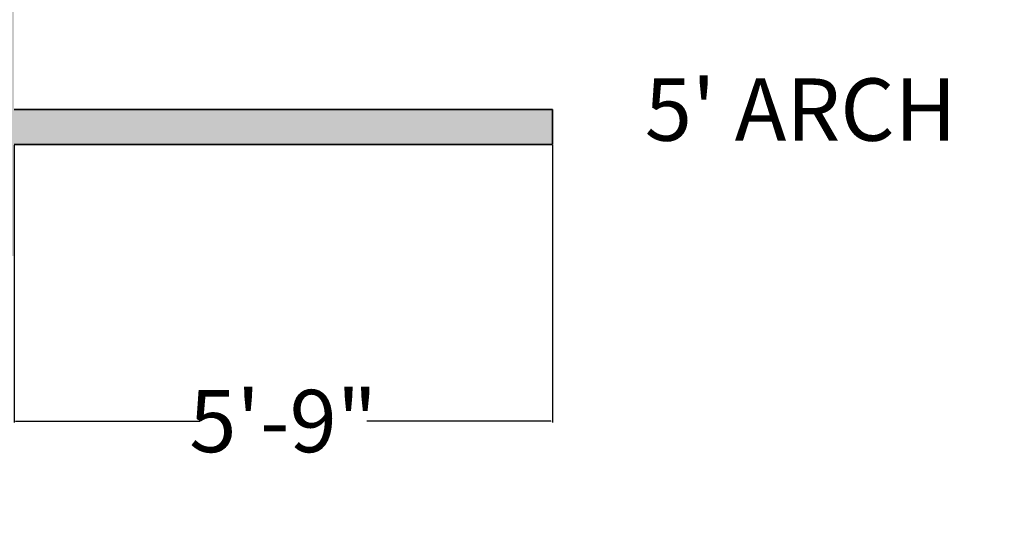
# Model space of a CAD drawing. Units: inches. Extents: x 638 to 1303, y 1 to 699.
# Tile 6 of 21: x 855 to 982, y 156 to 223. Entities that reach past the tile are written whole.
import ezdxf

# ---------------------------------------------------------------- set-up
doc = ezdxf.new("R2010")
doc.units = ezdxf.units.IN
doc.header["$MEASUREMENT"] = 0
for name, color, linetype, lineweight in [('A-ANNO-DIMS', 2, 'Continuous', 18), ('A-ANNO-TEXT', 7, 'Continuous', 18), ('A-WALL', 7, 'Continuous', 35)]:
    doc.layers.add(name, color=color, linetype=linetype, lineweight=lineweight)
doc.layers.add('A-WALL-PATT', color=143, linetype='Continuous', lineweight=13, true_color=0x7aafdf)
doc.styles.get("Standard").update_dxf_attribs({"font": 'arial.ttf'})
doc.dimstyles.get("Standard").update_dxf_attribs({"dimtxt": 8, "dimasz": 0.18, "dimexe": 0.18, "dimexo": 0.0625, "dimgap": 0.09, "dimtad": 0, "dimtih": 1, "dimtoh": 1, "dimdec": 4, "dimzin": 0, "dimdsep": 46, "dimlunit": 3, "dimtxsty": 'Standard', "dimcen": 0.09, "dimadec": 0, "dimazin": 0, "dimtfac": 1, "dimtdec": 4, "dimtofl": 0, "dimtmove": 0, "dimatfit": 3, "dimfxl": 1, "dimtolj": 1, "dimtzin": 0, "dimarcsym": 0})

# ---------------------------------------------------------------- blocks, each defined once
blk = doc.blocks.new('*D61')
at = {"layer": 'A-ANNO-DIMS', "color": 0, "lineweight": -2, "transparency": 16777216}
for p, q in [((854.74, 206.76), (854.74, 171.14)), ((923.85, 206.76), (923.85, 171.14)), ((854.92, 171.32), (878.57, 171.32)), ((923.67, 171.32), (900.02, 171.32))]:
    blk.add_line(p, q, dxfattribs=at)
at = {"layer": 'A-ANNO-DIMS', "color": 0, "transparency": 16777216}
for points in [[(854.92, 171.35), (854.92, 171.29), (854.74, 171.32)], [(923.67, 171.35), (923.67, 171.29), (923.85, 171.32)]]:
    blk.add_solid(points, dxfattribs=at)
at = {"layer": 'Defpoints', "color": 0, "transparency": 16777216}
for p in [(854.74, 206.82), (923.85, 206.82), (854.74, 171.32)]:
    blk.add_point(p, dxfattribs=at)
at = {"layer": 'A-ANNO-DIMS', "color": 0, "transparency": 16777216, "insert": (889.29, 171.32), "char_height": 8, "attachment_point": 5}
blk.add_mtext('\\A1;5\'-9"', dxfattribs=at)

msp = doc.modelspace()

# ---------------------------------------------------------------- hatches: boundary and pattern name
at = {"layer": 'A-WALL-PATT'}
h = msp.add_hatch(color=256, dxfattribs=at)
h.dxf.hatch_style = 1
h.paths.add_polyline_path([(973.34524, 629.81895), (793.35541, 629.81895), (793.35541, 620.81895), (850.23798, 620.81895), (922.23798, 620.81895), (922.23798, 524.81895), (908.94335, 524.81895), (908.94335, 520.31895), (926.73798, 520.31895), (926.73798, 544.31895), (979.3571, 544.31895), (979.3571, 548.81895), (926.73798, 548.81895), (926.73798, 620.81895), (973.34524, 620.81895)])
h.paths.add_polyline_path([(758.35541, 629.81895), (697.23798, 629.81895), (697.23798, 586.77451), (706.23798, 586.77451), (706.23798, 620.81895), (758.35541, 620.81895)])
h.paths.add_polyline_path([(1075.85281, 629.81895), (1003.34524, 629.81895), (1003.34524, 620.81895), (1046.73798, 620.81895), (1046.73798, 560.81895), (1046.73798, 548.81895), (1026.3571, 548.81895), (1026.3571, 544.31895), (1046.73798, 544.31895), (1046.73798, 486.87457), (1051.23798, 486.87457), (1051.23798, 556.31895), (1162.89753, 556.31895), (1162.89753, 560.81895), (1051.23798, 560.81895), (1051.23798, 620.81895), (1075.85281, 620.81895)])
h.paths.add_polyline_path([(1228.23798, 629.81895), (1105.85281, 629.81895), (1105.85281, 620.81895), (1219.23798, 620.81895), (1219.23798, 560.81895), (1197.89753, 560.81895), (1197.89753, 556.31895), (1219.23798, 556.31895), (1219.23798, 498.80084), (1228.23798, 498.80084)])
h.paths.add_polyline_path([(1051.23798, 439.87457), (1046.73798, 439.87457), (1046.73798, 407.81895), (1219.23798, 407.81895), (1219.23798, 381.66175), (1228.23798, 381.66175), (1228.23798, 451.80084), (1219.23798, 451.80084), (1219.23798, 412.31895), (1051.23798, 412.31895)])
h.paths.add_polyline_path([(1228.23798, 346.66175), (1219.23798, 346.66175), (1219.23798, 335.81895), (1046.73798, 335.81895), (1046.73798, 273.56895), (1051.23798, 273.56895), (1051.23798, 331.31895), (1219.23798, 331.31895), (1219.23798, 308.99654), (1228.23798, 308.99654)])
h.paths.add_polyline_path([(1228.23798, 261.99654), (1219.23798, 261.99654), (1219.23798, 211.31895), (1051.23798, 211.31895), (1051.23798, 226.56895), (1046.73798, 226.56895), (1046.73798, 211.31895), (983.84714, 211.31895), (983.84714, 206.81895), (1219.23798, 206.81895), (1219.23798, 166.83987), (1228.23798, 166.83987)])
h.paths.add_polyline_path([(1228.23798, 119.83987), (1219.23798, 119.83987), (1219.23798, 50.81895), (1197.89277, 50.81895), (1197.89277, 41.81895), (1228.23798, 41.81895)])
h.paths.add_polyline_path([(1162.89277, 50.81895), (1069.02949, 50.81895), (1069.02949, 41.81895), (1162.89277, 41.81895)])
h.paths.add_polyline_path([(1010.02949, 50.81895), (941.89631, 50.81895), (917.77455, 50.81895), (917.77455, 41.81895), (941.89631, 41.81895), (1010.02949, 41.81895)])
h.paths.add_polyline_path([(882.77455, 50.81895), (854.73798, 50.81895), (854.73798, 145.50379), (850.23798, 145.50379), (850.23798, 50.81895), (793.49755, 50.81895), (793.49755, 41.81895), (882.77455, 41.81895)])
h.paths.add_polyline_path([(746.49755, 50.81895), (706.23798, 50.81895), (706.23798, 96.57416), (697.23798, 96.57416), (697.23798, 41.81895), (746.49755, 41.81895)])
h.paths.add_polyline_path([(706.23798, 206.81895), (714.01165, 206.81895), (714.01165, 211.31895), (706.23798, 211.31895), (706.23798, 251.21966), (697.23798, 251.21966), (697.23798, 143.57416), (706.23798, 143.57416)])
h.paths.add_polyline_path([(923.84714, 211.31895), (854.73798, 211.31895), (854.73798, 397.8313), (850.23798, 397.8313), (850.23798, 388.31895), (747.9539, 388.31895), (747.9539, 383.81895), (850.23798, 383.81895), (850.23798, 311.81895), (706.23798, 311.81895), (706.23798, 342.78787), (697.23798, 342.78787), (697.23798, 281.21966), (706.23798, 281.21966), (706.23798, 307.31895), (850.23798, 307.31895), (850.23798, 211.31895), (749.01165, 211.31895), (749.01165, 206.81895), (850.23798, 206.81895), (850.23798, 192.50379), (854.73798, 192.50379), (854.73798, 206.81895), (923.84714, 206.81895)])
h.paths.add_polyline_path([(706.23798, 434.70471), (697.23798, 434.70471), (697.23798, 372.78787), (706.23798, 372.78787), (706.23798, 383.81895), (712.9539, 383.81895), (712.9539, 388.31895), (706.23798, 388.31895)])
h.paths.add_polyline_path([(706.23798, 520.31895), (850.23798, 520.31895), (850.23798, 444.8313), (854.73798, 444.8313), (854.73798, 520.31895), (861.94335, 520.31895), (861.94335, 524.81895), (706.23798, 524.81895), (706.23798, 551.77451), (697.23798, 551.77451), (697.23798, 481.70471), (706.23798, 481.70471)])

# ---------------------------------------------------------------- linework, layer by layer
at = {"layer": 'A-WALL'}
for p, q in [((923.84714, 211.31895), (854.73798, 211.31895)), ((923.84714, 211.31895), (923.84714, 206.81895)), ((923.84714, 206.81895), (854.73798, 206.81895))]:
    msp.add_line(p, q, dxfattribs=at)

# ---------------------------------------------------------------- texts
at = {"layer": 'A-ANNO-TEXT'}
msp.add_text("5' ARCH", height=8, dxfattribs=at).set_placement((935.72052, 207.31169))

# ---------------------------------------------------------------- dimensions: what is measured, and where the dimension line sits
at = {"layer": 'A-ANNO-DIMS'}
dim = msp.add_linear_dim(base=(854.73798, 171.31895), p1=(923.84714, 206.81895), p2=(854.73798, 206.81895), angle=180, dimstyle='Standard', override={"dimdec": 1, "dimlfac": 1, "dimrnd": 0, "dimzin": 1, "dimdsep": 46, "dimlunit": 4, "dimfrac": 2}, dxfattribs=at)
dim.commit()
dim.dimension.update_dxf_attribs({"geometry": '*D61', "text_midpoint": (889.29256, 171.31895)})

doc.saveas('drawing.dxf')
